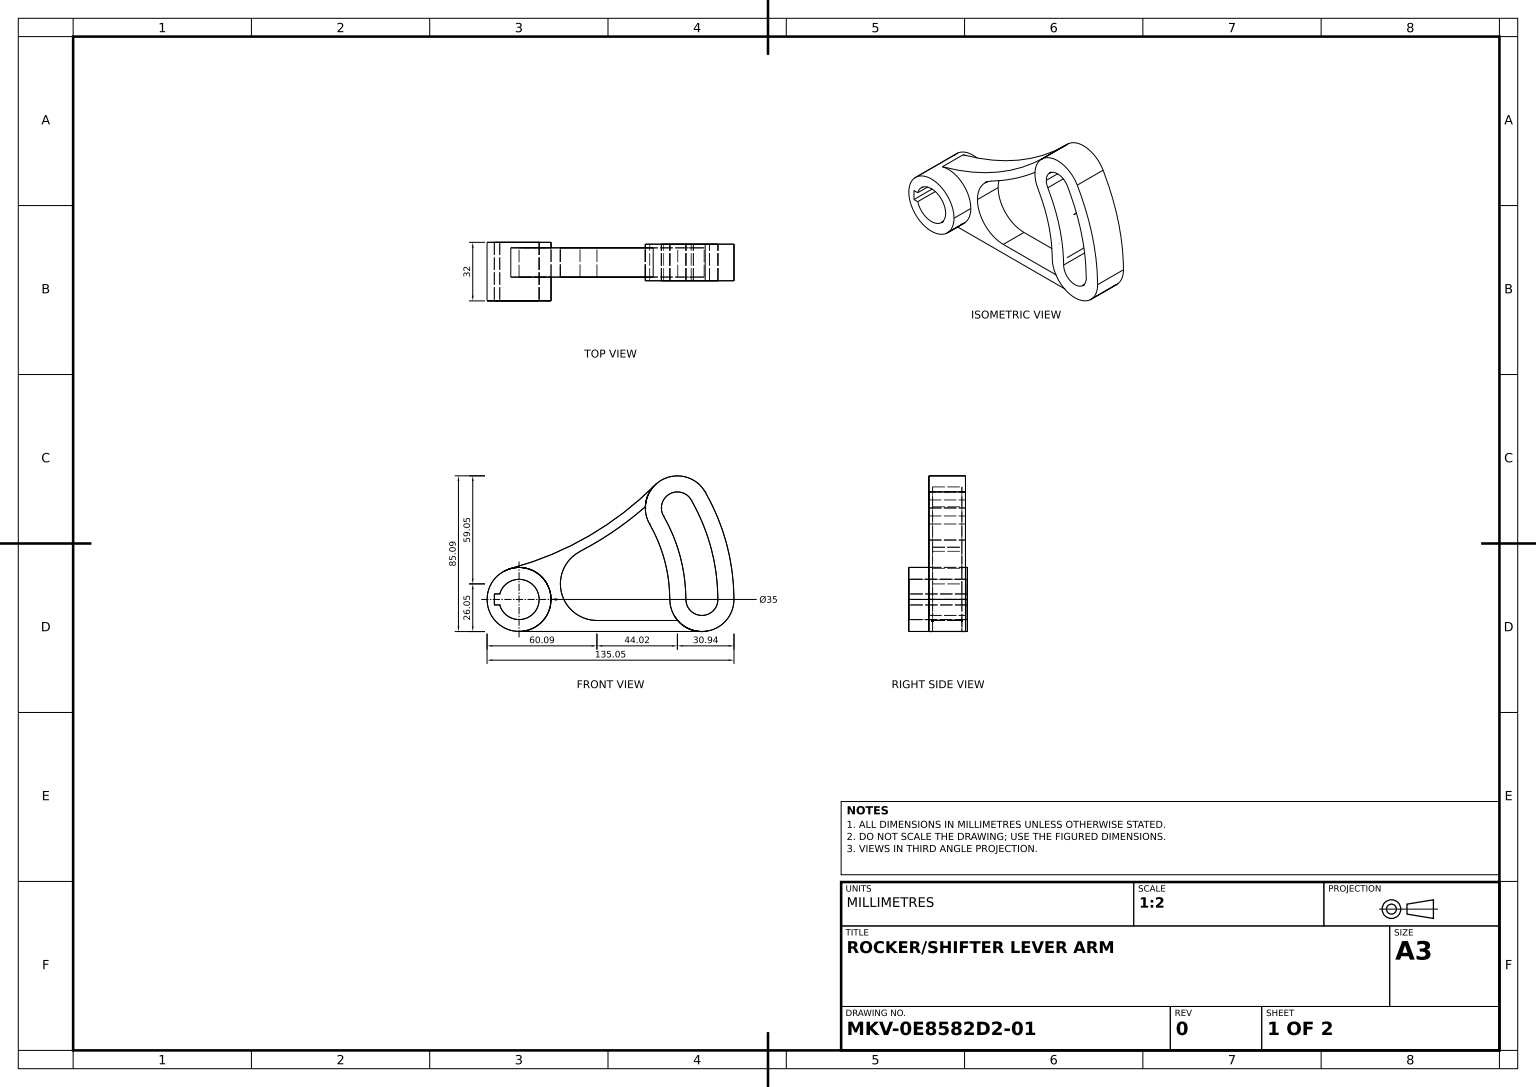
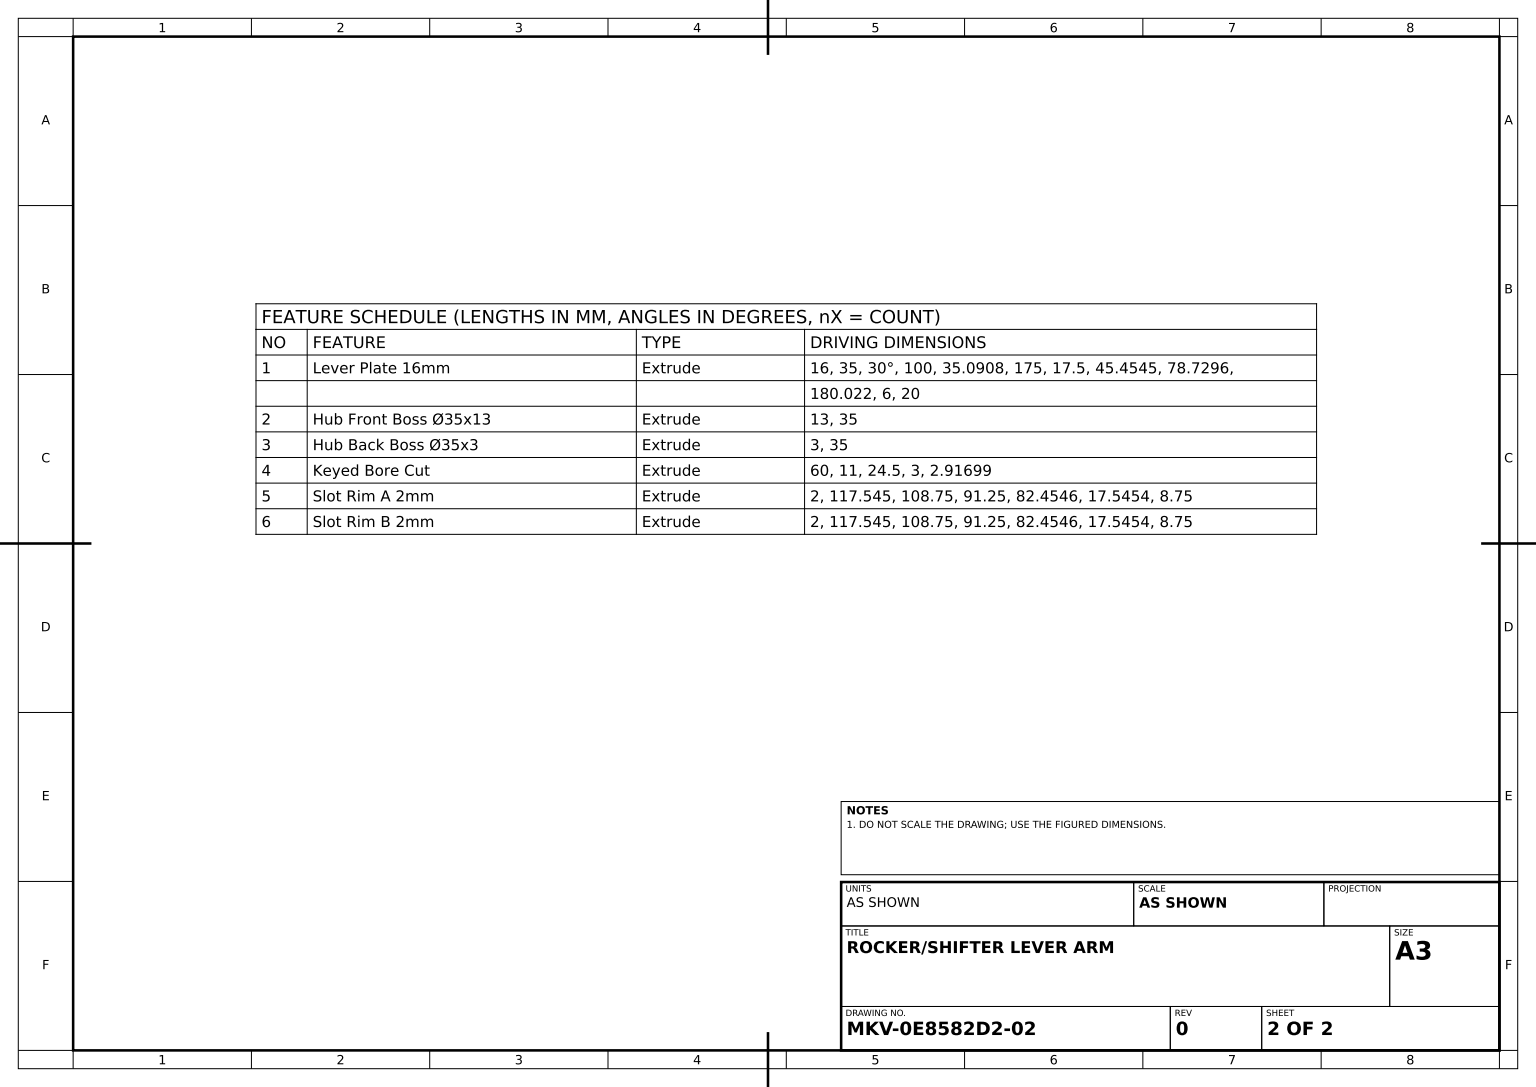
SolidWorks part; units mm, degrees
material "Plain Carbon Steel"
ref_plane "Front Plane" through (0, 0, 0) normal (0, 0, 1) x (1, 0, 0)
ref_plane "Top Plane" through (0, 0, 0) normal (0, 1, 0) x (1, 0, 0)
ref_plane "Right Plane" through (0, 0, 0) normal (1, 0, 0) x (0, 0, -1)
sketch "Lever Profile Sketch" plane through (0, 0, 0) normal (0, 0, 1) x (1, 0, 0)
  line L0 (82.4546, 0) -> (100, 0)
  line L1 (71.4078, 41.2273) -> (86.6025, 50)
  line L2 (0, -17.5) -> (101.2616, -17.5)
  line L3 (42.5862, -11.5) -> (86.7489, -11.5)
  arc A0 (-4.5132, 16.908) -> (0, -17.5) centre (0, 0) ccw
  arc A11 (100, 0) -> (86.6025, 50) centre (0, 0) ccw
  arc A12 (82.4546, 0) -> (117.5454, 0) centre (100, 0) ccw
  arc A14 (-4.5132, 16.908) -> (74.2164, 62.3626) centre (-49.6453, 185.9882) ccw
  arc A15 (94.1803, 54.375) -> (79.0248, 45.625) centre (86.6025, 50) ccw
  arc A16 (91.25, 0) -> (108.75, 0) centre (100, 0) ccw
  arc A17 (108.75, 0) -> (94.1803, 54.375) centre (0, 0) ccw
  arc A18 (91.25, 0) -> (79.0248, 45.625) centre (0, 0) ccw
  arc A19 (117.5454, 0) -> (101.7973, 58.7727) centre (0, 0) ccw
  arc A20 (82.4546, 0) -> (71.4078, 41.2273) centre (0, 0) ccw
  arc A21 (101.7973, 58.7727) -> (71.4078, 41.2273) centre (86.6025, 50) ccw
  arc A23 (33.3641, 26.2469) -> (69.0694, 50.6565) centre (-49.6453, 185.9882) ccw
  circle A24 centre (0, 0) radius 17.5
  arc A25 (33.3641, 26.2469) -> (42.5862, -11.5) centre (42.5862, 8.5) ccw
  dimension "D1" = 35
  dimension "D2" = 100
  dimension "D4" = 35.0908
  dimension "D5" = 45.4545
  dimension "D6" = 175
  dimension "D7" = 78.7296
  dimension "D8" = 17.5
  dimension "D9" = 20
  dimension "D10" = 180.0217
  dimension "D11" = 6
  dimension "D3" = 30
extrude "Lever Plate 16mm" add sketch "Lever Profile Sketch" along normal blind 16
sketch "Hub Front Sketch Ø35" plane through (0, 0, 16) normal (0, 0, 1) x (1, 0, 0)
  circle A0 centre (0, 0) radius 17.5
  dimension "D1" = 35
extrude "Hub Front Boss Ø35x13" add sketch "Hub Front Sketch Ø35" along normal blind 13
sketch "Hub Back Sketch Ø35" plane through (0, 0, 0) normal (0, 0, -1) x (-1, 0, 0)
  circle A0 centre (0, 0) radius 17.5
  dimension "D1" = 35
extrude "Hub Back Boss Ø35x3" add sketch "Hub Back Sketch Ø35" along normal blind 3
sketch "Keyed Bore Sketch" plane through (0, 0, 29) normal (0, 0, 1) x (1, 0, 0)
  line L0 (11, 0) -> (-13.5, 0)
  line L1 (-13.5, 0) -> (-13.5, 3)
  line L2 (-13.5, 3) -> (-10.583, 3)
  line L4 (-10.583, -3) -> (-13.5, -3)
  line L5 (-13.5, -3) -> (-13.5, 0)
  arc A0 (-10.583, -3) -> (-10.583, 3) centre (0, 0) ccw
  dimension "D1" = 11
  dimension "D2" = 24.5
  dimension "D3" = 3
  dimension "D4" = 2.917
extrude "Keyed Bore Cut" cut sketch "Keyed Bore Sketch" against normal blind 60 contours L4 A0 L0 L5 | L0 A0 L2 L1
sketch "Slot Rim Sketch A" plane through (0, 0, 16) normal (0, 0, 1) x (1, 0, 0)
  arc A0 (117.5454, 0) -> (101.7973, 58.7727) centre (0, 0) ccw
  arc A1 (108.75, 0) -> (94.1803, 54.375) centre (0, 0) ccw
  arc A2 (91.25, 0) -> (79.0248, 45.625) centre (0, 0) ccw
  arc A3 (82.4546, 0) -> (71.4078, 41.2273) centre (0, 0) ccw
  arc A4 (101.7973, 58.7727) -> (71.4078, 41.2273) centre (86.6025, 50) ccw
  arc A5 (94.1803, 54.375) -> (79.0248, 45.625) centre (86.6025, 50) ccw
  arc A6 (82.4546, 0) -> (117.5454, 0) centre (100, 0) ccw
  arc A7 (91.25, 0) -> (108.75, 0) centre (100, 0) ccw
  dimension "D1" = 117.5454
  dimension "D2" = 108.75
  dimension "D3" = 91.25
  dimension "D4" = 82.4546
  dimension "D5" = 17.5454
  dimension "D6" = 8.75
  dimension "D7" = 17.5454
  dimension "D8" = 8.75
extrude "Slot Rim A 2mm" add sketch "Slot Rim Sketch A" along normal blind 2
sketch "Slot Rim Sketch B" plane through (0, 0, 0) normal (0, 0, -1) x (-1, 0, 0)
  arc A0 (-101.7973, 58.7727) -> (-117.5454, 0) centre (0, 0) ccw
  arc A1 (-94.1803, 54.375) -> (-108.75, 0) centre (0, 0) ccw
  arc A2 (-79.0248, 45.625) -> (-91.25, 0) centre (0, 0) ccw
  arc A3 (-71.4078, 41.2273) -> (-82.4546, 0) centre (0, 0) ccw
  arc A4 (-71.4078, 41.2273) -> (-101.7973, 58.7727) centre (-86.6025, 50) ccw
  arc A5 (-117.5454, 0) -> (-82.4546, 0) centre (-100, 0) ccw
  arc A6 (-79.0248, 45.625) -> (-94.1803, 54.375) centre (-86.6025, 50) ccw
  arc A7 (-108.75, 0) -> (-91.25, 0) centre (-100, 0) ccw
  dimension "D1" = 117.5454
  dimension "D2" = 108.75
  dimension "D3" = 91.25
  dimension "D4" = 82.4546
  dimension "D5" = 17.5454
  dimension "D6" = 8.75
  dimension "D7" = 17.5454
  dimension "D8" = 8.75
extrude "Slot Rim B 2mm" add sketch "Slot Rim Sketch B" along normal blind 2
